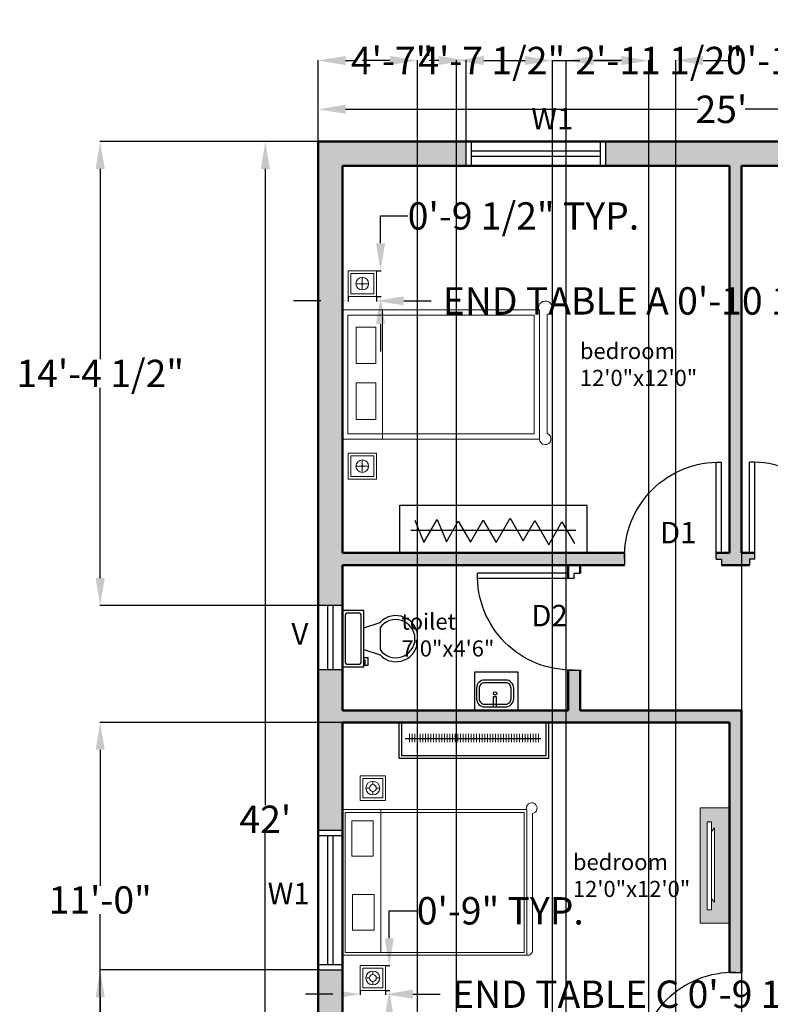
# Model space of a CAD drawing. Units: inches. Extents: x 2391 to 2964, y 130 to 798.
# Tile 3 of 4: x 2391 to 2671, y 431 to 798. Entities that reach past the tile are written whole.
import ezdxf

# ---------------------------------------------------------------- set-up
doc = ezdxf.new("R2010")
doc.units = ezdxf.units.IN
doc.header["$MEASUREMENT"] = 0
for name, color, linetype, lineweight in [('A-ANNO-DIMS', 2, 'Continuous', 18), ('A-ANNO-TEXT', 7, 'Continuous', 18), ('A-AREA-IDEN', 7, 'Continuous', 25), ('A-DOOR', 3, 'Continuous', 25), ('A-FLOR-CASE', 8, 'Continuous', 25), ('A-FLOR-CASE-PATT', 8, 'Continuous', 13), ('A-FLOR-FIXT', 9, 'Continuous', 25), ('A-FURN', 8, 'Continuous', 18), ('A-FURN-PATT', 8, 'Continuous', 13), ('A-GLAZ', 4, 'Continuous', 25), ('A-WALL', 7, 'Continuous', 50)]:
    doc.layers.add(name, color=color, linetype=linetype, lineweight=lineweight)
doc.layers.add('A-WALL-PATT', color=11, linetype='Continuous', lineweight=13, true_color=0xf27172)
doc.styles.get("Standard").update_dxf_attribs({"font": 'arial.ttf'})
doc.dimstyles.get("Standard").update_dxf_attribs({"dimtxt": 10.18, "dimasz": 10.18, "dimexe": 0.18, "dimexo": 0.0625, "dimgap": 0.09, "dimtad": 0, "dimtih": 1, "dimtoh": 1, "dimdec": 0, "dimzin": 0, "dimdsep": 46, "dimlunit": 3, "dimtxsty": 'Standard', "dimcen": 0.09, "dimadec": 0, "dimazin": 0, "dimtfac": 1, "dimtdec": 0, "dimtofl": 0, "dimtmove": 0, "dimatfit": 3, "dimfxl": 1, "dimtolj": 1, "dimtzin": 0, "dimarcsym": 0})

# ---------------------------------------------------------------- blocks, each defined once
blk = doc.blocks.new('*U2')
for p, q in [((9.5, -6), (9.5, -2)), ((-10, -8.5), (-8, -8.5)), ((-10, -9.5), (-10, -8.5)), ((-7, -9.5), (-10, -9.5)), ((-8, -8.5), (-8, -8)), ((-7, -8), (-7, -9.5)), ((-4, -8), (-6, -14)), ((4, -8), (6, -14)), ((4, -14), (-4, -14))]:
    blk.add_line(p, q)
blk.add_lwpolyline([(10.5, -8), (10.5, 0), (-10.5, 0), (-10.5, -8)], close=True)
for points in [[(-9.5, -2), (-9.5, -6)], [(8.5, -1), (-8.5, -1)], [(-8.5, -7), (8.5, -7)]]:
    blk.add_lwpolyline(points)
for centre, radius, start, end in [((-8.625, -1.875), 0.8839, 81.8699, 188.1301), ((8.625, -1.875), 0.8839, 351.8699, 98.1301), ((-8.625, -6.125), 0.8839, 171.869898, 278.1301), ((8.625, -6.125), 0.8839, 261.8699, 8.1301), ((-0.4772, -19.9188), 8.0953, 133.01722, 273.38), ((0.0374, -19.8731), 7.127, 124.50543, 269.7), ((-0.0373, -19.8731), 7.127, 270.3, 55.4946), ((0.4773, -19.9188), 8.0953, 266.62, 46.9828)]:
    blk.add_arc(centre, radius, start, end)
blk = doc.blocks.new('*D3')
at = {"layer": 'A-ANNO-DIMS', "color": 0, "lineweight": -2, "transparency": 16777216}
for p, q in [((2502.4, 752.3), (2502.4, 764.38)), ((2512.58, 764.2), (2643.58, 764.2)), ((2792.22, 764.2), (2661.21, 764.2)), ((2802.4, 752.3), (2802.4, 764.38))]:
    blk.add_line(p, q, dxfattribs=at)
at = {"layer": 'A-ANNO-DIMS', "color": 0, "transparency": 16777216}
for points in [[(2512.58, 765.89), (2512.58, 762.5), (2502.4, 764.2)], [(2792.22, 765.89), (2792.22, 762.5), (2802.4, 764.2)]]:
    blk.add_solid(points, dxfattribs=at)
at = {"layer": 'Defpoints', "color": 0, "transparency": 16777216}
for p in [(2802.4, 764.2), (2502.4, 752.24), (2802.4, 752.24)]:
    blk.add_point(p, dxfattribs=at)
at = {"layer": 'A-ANNO-DIMS', "color": 0, "transparency": 16777216, "insert": (2652.4, 764.2), "char_height": 10.18, "attachment_point": 5}
blk.add_mtext("\\A1;25'", dxfattribs=at)
blk = doc.blocks.new('*D4')
at = {"layer": 'A-ANNO-DIMS', "color": 0, "lineweight": -2, "transparency": 16777216}
for p, q in [((2502.34, 752.24), (2482.55, 752.24)), ((2482.73, 742.06), (2482.73, 505.44)), ((2482.73, 258.42), (2482.73, 495.03)), ((2502.34, 248.24), (2482.55, 248.24))]:
    blk.add_line(p, q, dxfattribs=at)
at = {"layer": 'A-ANNO-DIMS', "color": 0, "transparency": 16777216}
for points in [[(2481.03, 742.06), (2484.43, 742.06), (2482.73, 752.24)], [(2481.03, 258.42), (2484.43, 258.42), (2482.73, 248.24)]]:
    blk.add_solid(points, dxfattribs=at)
at = {"layer": 'Defpoints', "color": 0, "transparency": 16777216}
for p in [(2502.4, 752.24), (2482.73, 248.24), (2502.4, 248.24)]:
    blk.add_point(p, dxfattribs=at)
at = {"layer": 'A-ANNO-DIMS', "color": 0, "transparency": 16777216, "insert": (2482.73, 500.24), "char_height": 10.18, "attachment_point": 5}
blk.add_mtext("\\A1;42'", dxfattribs=at)
blk = doc.blocks.new('WIN-W1-48')
for p, q in [((0, 0), (0, 9)), ((2, 0), (2, 9)), ((50, 0), (50, 9)), ((52, 0), (52, 9)), ((2, 5.5), (50, 5.5)), ((2, 3.5), (50, 3.5))]:
    blk.add_line(p, q)
blk = doc.blocks.new('VENT-24')
for p, q in [((9, 24), (0, 24)), ((3.5, 24), (3.5, 0)), ((5.5, 24), (5.5, 0)), ((9, 0), (0, 0))]:
    blk.add_line(p, q)
blk = doc.blocks.new('DOOR-SWING-36')
for p, q in [((0, 4.5), (0, 38.25)), ((2, 2.25), (2, 38.25)), ((36, 4.5), (36, 0)), ((0, 2.25), (0, 0)), ((2, 2.25), (0, 2.25))]:
    blk.add_line(p, q)
blk.add_arc((1, 3.25), 35.01, 358.3634, 91.6366)
blk = doc.blocks.new('NIGHTSTAND-A')
for p, q in [((4.94, 4.82), (2.87, 4.82)), ((5.23, 5.11), (5.23, 7.18)), ((5.23, 4.53), (5.23, 2.47)), ((5.52, 4.82), (7.58, 4.82))]:
    blk.add_line(p, q)
for points in [[(0, 9.65), (10.46, 9.65), (10.46, 0), (0, 0)], [(1, 8.65), (9.46, 8.65), (9.46, 1), (1, 1)]]:
    blk.add_lwpolyline(points, close=True)
for radius in [2.35, 0.289]:
    blk.add_circle((5.23, 4.82), radius)
blk = doc.blocks.new('NIGHTSTAND-C')
for p, q in [((3.43, 4.62), (2.14, 4.62)), ((4.7, 5.9), (4.7, 7.18)), ((5.98, 4.62), (7.27, 4.62)), ((4.7, 3.34), (4.7, 2.06))]:
    blk.add_line(p, q)
for points in [[(0, 9.24), (9.41, 9.24), (9.41, 0), (0, 0)], [(1, 8.24), (8.41, 8.24), (8.41, 1), (1, 1)]]:
    blk.add_lwpolyline(points, close=True)
for radius in [2.56, 1.28]:
    blk.add_circle((4.7, 4.62), radius)
blk = doc.blocks.new('*D21')
at = {"layer": 'A-ANNO-DIMS', "color": 0, "lineweight": -2, "transparency": 16777216}
for p, q in [((2503.4, 692.98), (2493.22, 692.98)), ((2513.58, 694.49), (2513.58, 692.8)), ((2524.04, 694.49), (2524.04, 692.8)), ((2534.22, 692.98), (2544.4, 692.98))]:
    blk.add_line(p, q, dxfattribs=at)
at = {"layer": 'A-ANNO-DIMS', "color": 0, "transparency": 16777216}
for points in [[(2503.4, 694.68), (2503.4, 691.28), (2513.58, 692.98)], [(2534.22, 694.68), (2534.22, 691.28), (2524.04, 692.98)]]:
    blk.add_solid(points, dxfattribs=at)
at = {"layer": 'Defpoints', "color": 0, "transparency": 16777216}
for p in [(2513.58, 694.55), (2524.04, 694.55), (2524.04, 692.98)]:
    blk.add_point(p, dxfattribs=at)
at = {"layer": 'A-ANNO-DIMS', "color": 0, "transparency": 16777216, "insert": (2639.27, 692.98), "char_height": 10.18, "attachment_point": 5}
blk.add_mtext('\\A1;END TABLE A 0\'-10 1/2" TYP.', dxfattribs=at)
blk = doc.blocks.new('*D22')
at = {"layer": 'A-ANNO-DIMS', "color": 0, "lineweight": -2, "transparency": 16777216}
for p, q in [((2525.6, 714.37), (2525.6, 724.55)), ((2525.6, 724.55), (2535.78, 724.55)), ((2524.1, 704.19), (2525.78, 704.19)), ((2524.1, 694.55), (2525.78, 694.55)), ((2525.6, 684.37), (2525.6, 674.19))]:
    blk.add_line(p, q, dxfattribs=at)
at = {"layer": 'A-ANNO-DIMS', "color": 0, "transparency": 16777216}
for points in [[(2523.91, 714.37), (2527.3, 714.37), (2525.6, 704.19)], [(2523.91, 684.37), (2527.3, 684.37), (2525.6, 694.55)]]:
    blk.add_solid(points, dxfattribs=at)
at = {"layer": 'Defpoints', "color": 0, "transparency": 16777216}
for p in [(2524.04, 704.19), (2525.6, 704.19), (2524.04, 694.55)]:
    blk.add_point(p, dxfattribs=at)
at = {"layer": 'A-ANNO-DIMS', "color": 0, "transparency": 16777216, "insert": (2578.76, 724.55), "char_height": 10.18, "attachment_point": 5}
blk.add_mtext('\\A1;0\'-9 1/2" TYP.', dxfattribs=at)
blk = doc.blocks.new('*D25')
at = {"layer": 'A-ANNO-DIMS', "color": 0, "lineweight": -2, "transparency": 16777216}
for p, q in [((2518.03, 436.55), (2518.03, 435.02)), ((2527.43, 436.55), (2527.43, 435.02)), ((2507.85, 435.2), (2497.67, 435.2)), ((2537.61, 435.2), (2547.79, 435.2))]:
    blk.add_line(p, q, dxfattribs=at)
at = {"layer": 'A-ANNO-DIMS', "color": 0, "transparency": 16777216}
for points in [[(2507.85, 436.9), (2507.85, 433.5), (2518.03, 435.2)], [(2537.61, 436.9), (2537.61, 433.5), (2527.43, 435.2)]]:
    blk.add_solid(points, dxfattribs=at)
at = {"layer": 'Defpoints', "color": 0, "transparency": 16777216}
for p in [(2518.03, 436.61), (2527.43, 436.61), (2527.43, 435.2)]:
    blk.add_point(p, dxfattribs=at)
at = {"layer": 'A-ANNO-DIMS', "color": 0, "transparency": 16777216, "insert": (2639.1, 435.2), "char_height": 10.18, "attachment_point": 5}
blk.add_mtext('\\A1;END TABLE C 0\'-9 1/2" TYP.', dxfattribs=at)
blk = doc.blocks.new('*D26')
at = {"layer": 'A-ANNO-DIMS', "color": 0, "lineweight": -2, "transparency": 16777216}
for p, q in [((2528.84, 456.03), (2528.84, 466.21)), ((2528.84, 466.21), (2539.02, 466.21)), ((2527.5, 445.85), (2529.02, 445.85)), ((2527.5, 436.61), (2529.02, 436.61)), ((2528.84, 426.43), (2528.84, 416.25))]:
    blk.add_line(p, q, dxfattribs=at)
at = {"layer": 'A-ANNO-DIMS', "color": 0, "transparency": 16777216}
for points in [[(2527.15, 456.03), (2530.54, 456.03), (2528.84, 445.85)], [(2527.15, 426.43), (2530.54, 426.43), (2528.84, 436.61)]]:
    blk.add_solid(points, dxfattribs=at)
at = {"layer": 'Defpoints', "color": 0, "transparency": 16777216}
for p in [(2527.43, 445.85), (2528.84, 445.85), (2527.43, 436.61)]:
    blk.add_point(p, dxfattribs=at)
at = {"layer": 'A-ANNO-DIMS', "color": 0, "transparency": 16777216, "insert": (2570.14, 466.21), "char_height": 10.18, "attachment_point": 5}
blk.add_mtext('\\A1;0\'-9" TYP.', dxfattribs=at)
blk = doc.blocks.new('*D33')
at = {"layer": 'A-ANNO-DIMS', "color": 0, "lineweight": -2, "transparency": 16777216}
for p, q in [((2659.9, 743.17), (2659.9, 145.07)), ((2793.4, 743.17), (2793.4, 145.07)), ((2670.08, 145.25), (2697.69, 145.25)), ((2783.22, 145.25), (2755.61, 145.25))]:
    blk.add_line(p, q, dxfattribs=at)
at = {"layer": 'A-ANNO-DIMS', "color": 0, "transparency": 16777216}
for points in [[(2670.08, 146.95), (2670.08, 143.56), (2659.9, 145.25)], [(2783.22, 146.95), (2783.22, 143.56), (2793.4, 145.25)]]:
    blk.add_solid(points, dxfattribs=at)
at = {"layer": 'Defpoints', "color": 0, "transparency": 16777216}
for p in [(2659.9, 743.24), (2793.4, 743.24), (2793.4, 145.25)]:
    blk.add_point(p, dxfattribs=at)
at = {"layer": 'A-ANNO-DIMS', "color": 0, "transparency": 16777216, "insert": (2726.65, 145.25), "char_height": 10.18, "attachment_point": 5}
blk.add_mtext('\\A1;11\'-1 1/2"', dxfattribs=at)
blk = doc.blocks.new('*D34')
at = {"layer": 'A-ANNO-DIMS', "color": 0, "lineweight": -2, "transparency": 16777216}
for p, q in [((2511.34, 536.24), (2421.12, 536.24)), ((2421.3, 526.06), (2421.3, 475.52)), ((2421.3, 414.42), (2421.3, 464.95)), ((2511.34, 404.24), (2421.12, 404.24))]:
    blk.add_line(p, q, dxfattribs=at)
at = {"layer": 'A-ANNO-DIMS', "color": 0, "transparency": 16777216}
for points in [[(2419.6, 526.06), (2423, 526.06), (2421.3, 536.24)], [(2419.6, 414.42), (2423, 414.42), (2421.3, 404.24)]]:
    blk.add_solid(points, dxfattribs=at)
at = {"layer": 'Defpoints', "color": 0, "transparency": 16777216}
for p in [(2421.3, 536.24), (2511.4, 536.24), (2511.4, 404.24)]:
    blk.add_point(p, dxfattribs=at)
at = {"layer": 'A-ANNO-DIMS', "color": 0, "transparency": 16777216, "insert": (2421.3, 470.24), "char_height": 10.18, "attachment_point": 5}
blk.add_mtext('\\A1;11\'-0"', dxfattribs=at)
blk = doc.blocks.new('*D37')
at = {"layer": 'A-ANNO-DIMS', "color": 0, "lineweight": -2, "transparency": 16777216}
for p, q in [((2502.4, 752.3), (2502.4, 782.52)), ((2512.58, 782.34), (2516.07, 782.34)), ((2547.22, 782.34), (2543.73, 782.34)), ((2557.4, 752.3), (2557.4, 782.52))]:
    blk.add_line(p, q, dxfattribs=at)
at = {"layer": 'A-ANNO-DIMS', "color": 0, "transparency": 16777216}
for points in [[(2512.58, 784.03), (2512.58, 780.64), (2502.4, 782.34)], [(2547.22, 784.03), (2547.22, 780.64), (2557.4, 782.34)]]:
    blk.add_solid(points, dxfattribs=at)
at = {"layer": 'Defpoints', "color": 0, "transparency": 16777216}
for p in [(2557.4, 782.34), (2502.4, 752.24), (2557.4, 752.24)]:
    blk.add_point(p, dxfattribs=at)
at = {"layer": 'A-ANNO-DIMS', "color": 0, "transparency": 16777216, "insert": (2529.9, 782.34), "char_height": 10.18, "attachment_point": 5}
blk.add_mtext('\\A1;4\'-7"', dxfattribs=at)
blk = doc.blocks.new('*D39')
at = {"layer": 'A-ANNO-DIMS', "color": 0, "lineweight": -2, "transparency": 16777216}
for p, q in [((2502.34, 444.24), (2421.12, 444.24)), ((2421.3, 434.06), (2421.3, 419.34)), ((2421.3, 393.92), (2421.3, 408.63)), ((2502.34, 383.74), (2421.12, 383.74))]:
    blk.add_line(p, q, dxfattribs=at)
at = {"layer": 'A-ANNO-DIMS', "color": 0, "transparency": 16777216}
for points in [[(2419.6, 434.06), (2423, 434.06), (2421.3, 444.24)], [(2419.6, 393.92), (2423, 393.92), (2421.3, 383.74)]]:
    blk.add_solid(points, dxfattribs=at)
at = {"layer": 'Defpoints', "color": 0, "transparency": 16777216}
for p in [(2421.3, 444.24), (2502.4, 444.24), (2502.4, 383.74)]:
    blk.add_point(p, dxfattribs=at)
at = {"layer": 'A-ANNO-DIMS', "color": 0, "transparency": 16777216, "insert": (2421.3, 413.99), "char_height": 10.18, "attachment_point": 5}
blk.add_mtext('\\A1;5\'-0 1/2"', dxfattribs=at)
blk = doc.blocks.new('*D40')
at = {"layer": 'A-ANNO-DIMS', "color": 0, "lineweight": -2, "transparency": 16777216}
for p, q in [((2502.34, 752.24), (2421.12, 752.24)), ((2421.3, 742.06), (2421.3, 671.34)), ((2421.3, 589.92), (2421.3, 660.63)), ((2502.34, 579.74), (2421.12, 579.74))]:
    blk.add_line(p, q, dxfattribs=at)
at = {"layer": 'A-ANNO-DIMS', "color": 0, "transparency": 16777216}
for points in [[(2419.6, 742.06), (2423, 742.06), (2421.3, 752.24)], [(2419.6, 589.92), (2423, 589.92), (2421.3, 579.74)]]:
    blk.add_solid(points, dxfattribs=at)
at = {"layer": 'Defpoints', "color": 0, "transparency": 16777216}
for p in [(2421.3, 752.24), (2502.4, 752.24), (2502.4, 579.74)]:
    blk.add_point(p, dxfattribs=at)
at = {"layer": 'A-ANNO-DIMS', "color": 0, "transparency": 16777216, "insert": (2421.3, 665.99), "char_height": 10.18, "attachment_point": 5}
blk.add_mtext('\\A1;14\'-4 1/2"', dxfattribs=at)
blk = doc.blocks.new('*D49')
at = {"layer": 'A-ANNO-DIMS', "color": 0, "lineweight": -2, "transparency": 16777216}
for p, q in [((2529.11, 782.34), (2518.93, 782.34)), ((2539.29, 342.63), (2539.29, 782.52)), ((2594.63, 342.63), (2594.63, 782.52)), ((2604.81, 782.34), (2614.99, 782.34))]:
    blk.add_line(p, q, dxfattribs=at)
at = {"layer": 'A-ANNO-DIMS', "color": 0, "transparency": 16777216}
for points in [[(2529.11, 784.03), (2529.11, 780.64), (2539.29, 782.34)], [(2604.81, 784.03), (2604.81, 780.64), (2594.63, 782.34)]]:
    blk.add_solid(points, dxfattribs=at)
at = {"layer": 'Defpoints', "color": 0, "transparency": 16777216}
for p in [(2594.63, 782.34), (2539.29, 342.57), (2594.63, 342.57)]:
    blk.add_point(p, dxfattribs=at)
at = {"layer": 'A-ANNO-DIMS', "color": 0, "transparency": 16777216, "insert": (2566.96, 782.34), "char_height": 10.18, "attachment_point": 5}
blk.add_mtext('\\A1;4\'-7 1/2"', dxfattribs=at)
blk = doc.blocks.new('*D52')
at = {"layer": 'A-ANNO-DIMS', "color": 0, "lineweight": -2, "transparency": 16777216}
for p, q in [((2615.22, 782.34), (2605.04, 782.34)), ((2625.4, 311.3), (2625.4, 782.52)), ((2635.4, 311.3), (2635.4, 782.52)), ((2645.58, 782.34), (2655.76, 782.34))]:
    blk.add_line(p, q, dxfattribs=at)
at = {"layer": 'A-ANNO-DIMS', "color": 0, "transparency": 16777216}
for points in [[(2615.22, 784.03), (2615.22, 780.64), (2625.4, 782.34)], [(2645.58, 784.03), (2645.58, 780.64), (2635.4, 782.34)]]:
    blk.add_solid(points, dxfattribs=at)
at = {"layer": 'Defpoints', "color": 0, "transparency": 16777216}
for p in [(2635.4, 782.34), (2625.4, 311.24), (2635.4, 311.24)]:
    blk.add_point(p, dxfattribs=at)
at = {"layer": 'A-ANNO-DIMS', "color": 0, "transparency": 16777216, "insert": (2673.33, 782.34), "char_height": 10.18, "attachment_point": 5}
blk.add_mtext('\\A1;0\'-10"', dxfattribs=at)
blk = doc.blocks.new('*D54')
at = {"layer": 'A-ANNO-DIMS', "color": 0, "lineweight": -2, "transparency": 16777216}
for p, q in [((2553.9, 335.07), (2553.9, 782.52)), ((2564.08, 782.34), (2579.34, 782.34)), ((2589.52, 335.07), (2589.52, 782.52)), ((2589.52, 782.34), (2599.7, 782.34))]:
    blk.add_line(p, q, dxfattribs=at)
at = {"layer": 'A-ANNO-DIMS', "color": 0, "transparency": 16777216}
for points in [[(2564.08, 784.03), (2564.08, 780.64), (2553.9, 782.34)], [(2579.34, 784.03), (2579.34, 780.64), (2589.52, 782.34)]]:
    blk.add_solid(points, dxfattribs=at)
at = {"layer": 'Defpoints', "color": 0, "transparency": 16777216}
for p in [(2589.52, 782.34), (2553.9, 335.01), (2589.52, 335.01)]:
    blk.add_point(p, dxfattribs=at)
at = {"layer": 'A-ANNO-DIMS', "color": 0, "transparency": 16777216, "insert": (2629.23, 782.34), "char_height": 10.18, "attachment_point": 5}
blk.add_mtext('\\A1;2\'-11 1/2"', dxfattribs=at)

msp = doc.modelspace()

# ---------------------------------------------------------------- hatches: boundary and pattern name
at = {"layer": 'A-FLOR-CASE-PATT'}
h = msp.add_hatch(dxfattribs=at)
h.set_pattern_fill('ANSI31', color=256, scale=8.001095, angle=45, style=0)
h.paths.add_polyline_path([(2536.34, 528.9), (2584.36, 528.9), (2584.36, 531.99), (2536.34, 531.99)])
at = {"layer": 'A-FURN-PATT'}
h = msp.add_hatch(color=256, dxfattribs=at)
h.dxf.hatch_style = 1
h.paths.add_polyline_path([(2648.69, 499.23), (2647.07, 499.23), (2647.07, 466.63), (2648.69, 466.63)], flags=16)
h.paths.add_polyline_path([(2655.4, 504.5), (2644.56, 504.5), (2644.56, 461.62), (2655.4, 461.62)])
h.paths.add_polyline_path([(2648.69, 470.61), (2649.84, 469.43), (2649.84, 497.04), (2648.69, 495.7)], flags=16)
at = {"layer": 'A-WALL-PATT'}
h = msp.add_hatch(color=256, dxfattribs=at)
h.dxf.hatch_style = 1
h.paths.add_polyline_path([(2557.4, 752.24), (2502.4, 752.24), (2502.4, 579.74), (2511.4, 579.74), (2511.4, 594.74), (2595.4, 594.74), (2599.9, 594.74), (2616.4, 594.74), (2616.4, 596.99, -0.014283), (2616.4, 598.99), (2616.4, 599.24), (2511.4, 599.24), (2511.4, 743.24), (2557.4, 743.24)])
h.paths.add_polyline_path([(2700.65, 752.24), (2609.4, 752.24), (2609.4, 743.24), (2655.4, 743.24), (2655.4, 599.24), (2650.4, 599.24), (2650.4, 596.99), (2652.4, 596.99), (2652.4, 594.74), (2662.9, 594.74), (2662.9, 596.99), (2664.9, 596.99), (2664.9, 599.24), (2659.9, 599.24), (2659.9, 743.24), (2700.65, 743.24)])
h.paths.add_polyline_path([(2802.4, 752.24), (2752.65, 752.24), (2752.65, 743.24), (2793.4, 743.24), (2793.4, 599.24), (2698.9, 599.24), (2698.9, 598.99, -0.014283), (2698.9, 596.99), (2698.9, 594.74), (2704.9, 594.74), (2704.9, 536.24), (2737.79, 536.24), (2737.79, 540.74), (2709.4, 540.74), (2709.4, 594.74), (2793.4, 594.74), (2793.4, 581.74), (2802.4, 581.74)])
h.paths.add_polyline_path([(2511.4, 444.24), (2502.4, 444.24), (2502.4, 383.74), (2511.4, 383.74), (2511.4, 399.74), (2655.4, 399.74), (2655.4, 354.74), (2655.65, 354.74, -0.014283), (2657.65, 354.74), (2659.9, 354.74), (2659.9, 407.24), (2657.65, 407.24), (2657.65, 409.24), (2655.4, 409.24), (2655.4, 404.24), (2511.4, 404.24)])
h.paths.add_polyline_path([(2511.4, 536.24), (2599.9, 536.24), (2655.4, 536.24), (2655.4, 443.24), (2655.65, 443.24, -0.014283), (2657.65, 443.24), (2659.9, 443.24), (2659.9, 540.74), (2599.9, 540.74), (2599.9, 555.74), (2597.65, 555.74, -0.014283), (2595.65, 555.74), (2595.4, 555.74), (2595.4, 540.74), (2511.4, 540.74), (2511.4, 555.74), (2502.4, 555.74), (2502.4, 496.24), (2511.4, 496.24), (2511.4, 503.82)])
h.paths.add_polyline_path([(2676.45, 257.24), (2511.4, 257.24), (2511.4, 311.24), (2659.9, 311.24), (2659.9, 318.74), (2657.65, 318.74), (2657.65, 320.74), (2655.4, 320.74), (2655.4, 315.74), (2511.4, 315.74), (2511.4, 331.74), (2502.4, 331.74), (2502.4, 248.24), (2676.45, 248.24)])
h.paths.add_polyline_path([(2802.4, 370.74), (2793.4, 370.74), (2793.4, 257.24), (2787.63, 257.24), (2787.63, 248.24), (2802.4, 248.24)])
h.paths.add_polyline_path([(2735.63, 257.24), (2715.45, 257.24), (2715.45, 254.74, -0.014283), (2715.45, 252.74), (2715.45, 248.24), (2721.55, 248.24), (2735.63, 248.24)])
h.paths.add_polyline_path([(2802.4, 553.74), (2793.4, 553.74), (2793.4, 540.74), (2763.73, 540.74), (2763.73, 536.24), (2793.4, 536.24), (2793.4, 422.74), (2802.4, 422.74)])

# ---------------------------------------------------------------- linework, layer by layer
at = {"layer": 'A-FLOR-CASE'}
for p, q in [((2532.74, 599.24), (2532.74, 617)), ((2532.74, 617), (2602.38, 617)), ((2602.38, 617), (2602.38, 599.24)), ((2538.4, 611.43), (2541.73, 603.2)), ((2541.73, 603.2), (2546.65, 611.72)), ((2546.65, 611.72), (2550.08, 603.41)), ((2559.06, 603.3), (2563.79, 611.5)), ((2563.79, 611.5), (2568.59, 603.19)), ((2568.59, 603.19), (2573.77, 612.16)), ((2573.77, 612.16), (2578.61, 603.78)), ((2536.88, 607.72), (2598.24, 607.72)), ((2550.08, 603.41), (2554.53, 611.13)), ((2554.53, 611.13), (2559.06, 603.3)), ((2578.61, 603.78), (2582.97, 611.33)), ((2582.97, 611.33), (2588.17, 602.33)), ((2588.17, 602.33), (2593.08, 610.84)), ((2593.08, 610.84), (2597.74, 602.76)), ((2532.36, 536.24), (2532.36, 522.95)), ((2533.36, 536.24), (2533.36, 523.95)), ((2587.22, 523.95), (2587.22, 536.24)), ((2588.22, 522.95), (2588.22, 536.24)), ((2534.71, 530.31), (2585.25, 530.31)), ((2533.36, 523.95), (2587.22, 523.95)), ((2532.36, 522.95), (2588.22, 522.95))]:
    msp.add_line(p, q, dxfattribs=at)
at = {"layer": 'A-FLOR-FIXT'}
for p, q in [((2560.67, 540.74), (2560.67, 555.11)), ((2560.67, 555.11), (2576.64, 555.11)), ((2576.64, 555.11), (2576.64, 540.74))]:
    msp.add_line(p, q, dxfattribs=at)
for points in [[(2561.31, 545.03, 0.414214), (2564.31, 542.03), (2572.13, 542.03, 0.414214), (2575.13, 545.03), (2575.13, 549.02, 0.414214), (2572.13, 552.02), (2564.31, 552.02, 0.414214), (2561.31, 549.02)], [(2562.31, 545.03, 0.414214), (2564.31, 543.03), (2572.13, 543.03, 0.414214), (2574.13, 545.03), (2574.13, 549.02, 0.414214), (2572.13, 551.02), (2564.31, 551.02, 0.414214), (2562.31, 549.02)]]:
    msp.add_lwpolyline(points, format="xyb", close=True, dxfattribs=at)
msp.add_lwpolyline([(2567.5, 542.03), (2567.5, 542.03), (2568.72, 542.03), (2568.72, 542.03), (2568.72, 545.79), (2568.72, 545.79), (2567.5, 545.79), (2567.5, 545.79)], close=True, dxfattribs=at)
msp.add_circle((2568.22, 547.03), 0.613, dxfattribs=at)
at = {"layer": 'A-FURN'}
for p, q in [((2526.3, 689.63), (2526.3, 641.6)), ((2587.54, 687.86), (2587.54, 643.72)), ((2525.75, 503.82), (2525.75, 450.77)), ((2582.13, 502.41), (2582.13, 451.5)), ((2648.69, 495.7), (2649.84, 497.04)), ((2649.84, 497.04), (2649.84, 469.43)), ((2649.84, 469.43), (2648.69, 470.61))]:
    msp.add_line(p, q, dxfattribs=at)
for points in [[(2511.4, 689.63), (2584.7, 689.63), (2584.7, 641.6), (2511.4, 641.6)], [(2513.4, 687.63), (2582.7, 687.63), (2582.7, 643.6), (2513.4, 643.6)], [(2516.57, 683.23), (2523.89, 683.23), (2523.89, 669.64), (2516.57, 669.64)], [(2516.57, 662.48), (2523.89, 662.48), (2523.89, 648.9), (2516.57, 648.9)], [(2511.4, 503.82), (2580.07, 503.82), (2580.07, 449.77), (2511.4, 449.77)], [(2512.4, 502.82), (2579.07, 502.82), (2579.07, 450.77), (2512.4, 450.77)], [(2655.4, 504.5), (2644.56, 504.5), (2644.56, 461.62), (2655.4, 461.62)], [(2514.88, 499.72), (2522.89, 499.72), (2522.89, 486.48), (2514.88, 486.48)], [(2648.69, 499.23), (2647.07, 499.23), (2647.07, 466.63), (2648.69, 466.63)], [(2515.16, 472.27), (2523.17, 472.27), (2523.17, 459.03), (2515.16, 459.03)]]:
    msp.add_lwpolyline(points, close=True, dxfattribs=at)
for centre, radius, start, end in [((2586.93, 690.36), 2.57, 283.6234, 196.3766), ((2586.86, 641.67), 2.16, 181.738, 71.7984), ((2581.84, 504.38), 1.99, 278.3608, 196.4357), ((2580.44, 451.42), 1.69, 257.4081, 2.4952)]:
    msp.add_arc(centre, radius, start, end, dxfattribs=at)
at = {"layer": 'A-WALL'}
for p, q in [((2502.4, 248.24), (2502.4, 752.24)), ((2502.4, 752.24), (2802.4, 752.24)), ((2511.4, 743.24), (2655.4, 743.24)), ((2511.4, 599.24), (2511.4, 743.24)), ((2655.4, 599.24), (2655.4, 743.24)), ((2659.9, 599.24), (2659.9, 743.24)), ((2659.9, 743.24), (2793.4, 743.24)), ((2511.4, 599.24), (2616.41, 599.24)), ((2650.4, 599.24), (2655.4, 599.24)), ((2659.9, 599.24), (2664.9, 599.24)), ((2511.4, 594.74), (2595.4, 594.74)), ((2511.4, 540.74), (2511.4, 594.74)), ((2595.4, 594.74), (2599.9, 594.74)), ((2595.4, 589.74), (2595.4, 594.74)), ((2599.9, 594.74), (2616.4, 594.74)), ((2599.9, 591.74), (2599.9, 594.74)), ((2652.4, 594.74), (2662.9, 594.74)), ((2595.4, 540.74), (2595.4, 555.74)), ((2599.9, 540.74), (2599.9, 555.74)), ((2511.4, 540.74), (2595.4, 540.74)), ((2511.4, 540.74), (2595.4, 540.74)), ((2599.9, 540.74), (2659.9, 540.74)), ((2659.9, 443.24), (2659.9, 540.74)), ((2659.9, 443.24), (2659.9, 540.74)), ((2511.4, 536.24), (2599.9, 536.24)), ((2511.4, 536.24), (2655.4, 536.24)), ((2511.4, 404.24), (2511.4, 536.24)), ((2655.4, 443.23), (2655.4, 536.24)), ((2655.4, 443.23), (2655.4, 536.24))]:
    msp.add_line(p, q, dxfattribs=at)

# ---------------------------------------------------------------- block references
at = {"layer": 'A-DOOR', "extrusion": (0, 0, -1), "zscale": -1}
msp.add_blockref('DOOR-SWING-36', (-2652.4, 594.74), dxfattribs=at)
at = {"layer": 'A-DOOR'}
msp.add_blockref('DOOR-SWING-36', (2662.9, 594.74), dxfattribs=at)
at = {"layer": 'A-DOOR', "extrusion": (0, 0, -1), "zscale": -1, "rotation": 270.0000000000014}
msp.add_blockref('DOOR-SWING-36', (-2599.9, 591.73), dxfattribs=at)
at = {"layer": 'A-DOOR', "rotation": 89.99999999999888}
msp.add_blockref('DOOR-SWING-36', (2659.9, 407.24), dxfattribs=at)
at = {"layer": 'A-FLOR-FIXT', "rotation": 90}
msp.add_blockref('*U2', (2511.4, 567.39), dxfattribs=at)
at = {"layer": 'A-FURN'}
for name, p in [('NIGHTSTAND-A', (2513.58, 694.55)), ('NIGHTSTAND-A', (2513.58, 626.7)), ('NIGHTSTAND-C', (2518.03, 507.21)), ('NIGHTSTAND-C', (2518.03, 436.61))]:
    msp.add_blockref(name, p, dxfattribs=at)
at = {"layer": 'A-GLAZ'}
for name, p in [('WIN-W1-48', (2557.4, 743.24)), ('VENT-24', (2502.4, 555.74))]:
    msp.add_blockref(name, p, dxfattribs=at)
at = {"layer": 'A-GLAZ', "rotation": 269.999999999996}
msp.add_blockref('WIN-W1-48', (2502.4, 496.23), dxfattribs=at)

# ---------------------------------------------------------------- texts
at = {"layer": 'A-ANNO-TEXT', "char_height": 8, "attachment_point": 1}
for s, insert in [('W1', (2581.67, 764.73)), ('D1', (2629.55, 610.81)), ('D2', (2581.66, 579.96)), ('V', (2492.45, 573.16)), ('W1', (2483.59, 476.67))]:
    msp.add_mtext_dynamic_manual_height_columns(s, width=35.9617, gutter_width=1, heights=[0], dxfattribs=dict(at, insert=insert))
at = {"layer": 'A-AREA-IDEN', "char_height": 6, "attachment_point": 1}
for s, insert in [('bedroom\\P12\'0"x12\'0"', (2599.76, 677.34)), ('toilet\\P7\'0"x4\'6"', (2533.37, 576.75)), ('bedroom\\P12\'0"x12\'0"', (2597.16, 487.34))]:
    msp.add_mtext_dynamic_manual_height_columns(s, width=87.7895, gutter_width=1, heights=[0], dxfattribs=dict(at, insert=insert))

# ---------------------------------------------------------------- dimensions: what is measured, and where the dimension line sits
at = {"layer": 'A-ANNO-DIMS'}
for base, p1, p2, override, picture, middle in [((2594.63, 782.34), (2539.29, 342.57), (2594.63, 342.57), {"dimdec": 1, "dimlfac": 1, "dimrnd": 0, "dimzin": 1, "dimdsep": 46, "dimlunit": 4, "dimfrac": 2}, '*D49', (2566.96, 782.34)), ((2589.52, 782.34), (2553.9, 335.01), (2589.52, 335.01), {"dimdec": 1, "dimlfac": 1, "dimrnd": 0, "dimzin": 1, "dimdsep": 46, "dimlunit": 4, "dimfrac": 2}, '*D54', (2629.23, 782.34)), ((2557.4, 782.34), (2502.4, 752.24), (2557.4, 752.24), {"dimdec": 1, "dimlfac": 1, "dimrnd": 0, "dimzin": 1, "dimdsep": 46, "dimlunit": 4, "dimfrac": 2}, '*D37', (2529.9, 782.34)), ((2635.4, 782.34), (2625.4, 311.24), (2635.4, 311.24), {"dimdec": 1, "dimlfac": 1, "dimrnd": 0, "dimzin": 1, "dimdsep": 46, "dimlunit": 4, "dimfrac": 2}, '*D52', (2673.33, 782.34)), ((2802.4, 764.2), (2502.4, 752.24), (2802.4, 752.24), {"dimclrd": 0, "dimclre": 0, "dimclrt": 0}, '*D3', (2652.4, 764.2)), ((2793.4, 145.25), (2659.9, 743.24), (2793.4, 743.24), {"dimdec": 1, "dimlfac": 1, "dimrnd": 0, "dimzin": 1, "dimdsep": 46, "dimlunit": 4, "dimfrac": 2}, '*D33', (2726.65, 145.25))]:
    dim = msp.add_linear_dim(base=base, p1=p1, p2=p2, dimstyle='Standard', override=override, dxfattribs=at)
    dim.commit()
    dim.dimension.update_dxf_attribs({"geometry": picture, "text_midpoint": middle})
for base, p1, p2, override, picture, middle in [((2421.3, 752.24), (2502.4, 579.74), (2502.4, 752.24), {"dimdec": 1, "dimlfac": 1, "dimrnd": 0, "dimzin": 1, "dimdsep": 46, "dimlunit": 4, "dimfrac": 2}, '*D40', (2421.3, 665.99)), ((2482.73, 248.24), (2502.4, 752.24), (2502.4, 248.24), {"dimclrd": 0, "dimclre": 0, "dimclrt": 0}, '*D4', (2482.73, 500.24)), ((2421.3, 536.24), (2511.4, 404.24), (2511.4, 536.24), {"dimdec": 1, "dimlfac": 1, "dimrnd": 0, "dimzin": 1, "dimdsep": 46, "dimlunit": 4, "dimfrac": 2}, '*D34', (2421.3, 470.24)), ((2421.3, 444.24), (2502.4, 383.74), (2502.4, 444.24), {"dimdec": 1, "dimlfac": 1, "dimrnd": 0, "dimzin": 1, "dimdsep": 46, "dimlunit": 4, "dimfrac": 2}, '*D39', (2421.3, 413.99))]:
    dim = msp.add_linear_dim(base=base, p1=p1, p2=p2, angle=90, dimstyle='Standard', override=override, dxfattribs=at)
    dim.commit()
    dim.dimension.update_dxf_attribs({"geometry": picture, "text_midpoint": middle})
for base, p1, p2, picture, middle in [((2525.6, 704.19), (2524.04, 694.55), (2524.04, 704.19), '*D22', (2578.76, 724.55)), ((2528.84, 445.85), (2527.43, 436.61), (2527.43, 445.85), '*D26', (2570.14, 466.21))]:
    dim = msp.add_linear_dim(base=base, p1=p1, p2=p2, angle=90, text='<> TYP.', dimstyle='Standard', override={"dimdec": 1, "dimlfac": 1, "dimrnd": 0, "dimzin": 1, "dimdsep": 46, "dimlunit": 4, "dimfrac": 2}, dxfattribs=at)
    dim.commit()
    dim.dimension.update_dxf_attribs({"geometry": picture, "text_midpoint": middle})
for base, p1, p2, text, picture, middle in [((2524.04, 692.98), (2513.58, 694.55), (2524.04, 694.55), 'END TABLE A <> TYP.', '*D21', (2639.27, 692.98)), ((2527.43, 435.2), (2518.03, 436.61), (2527.43, 436.61), 'END TABLE C <> TYP.', '*D25', (2639.1, 435.2))]:
    dim = msp.add_linear_dim(base=base, p1=p1, p2=p2, text=text, dimstyle='Standard', override={"dimdec": 1, "dimlfac": 1, "dimrnd": 0, "dimzin": 1, "dimdsep": 46, "dimlunit": 4, "dimfrac": 2}, dxfattribs=at)
    dim.commit()
    dim.dimension.update_dxf_attribs({"geometry": picture, "text_midpoint": middle})

doc.saveas('drawing.dxf')
